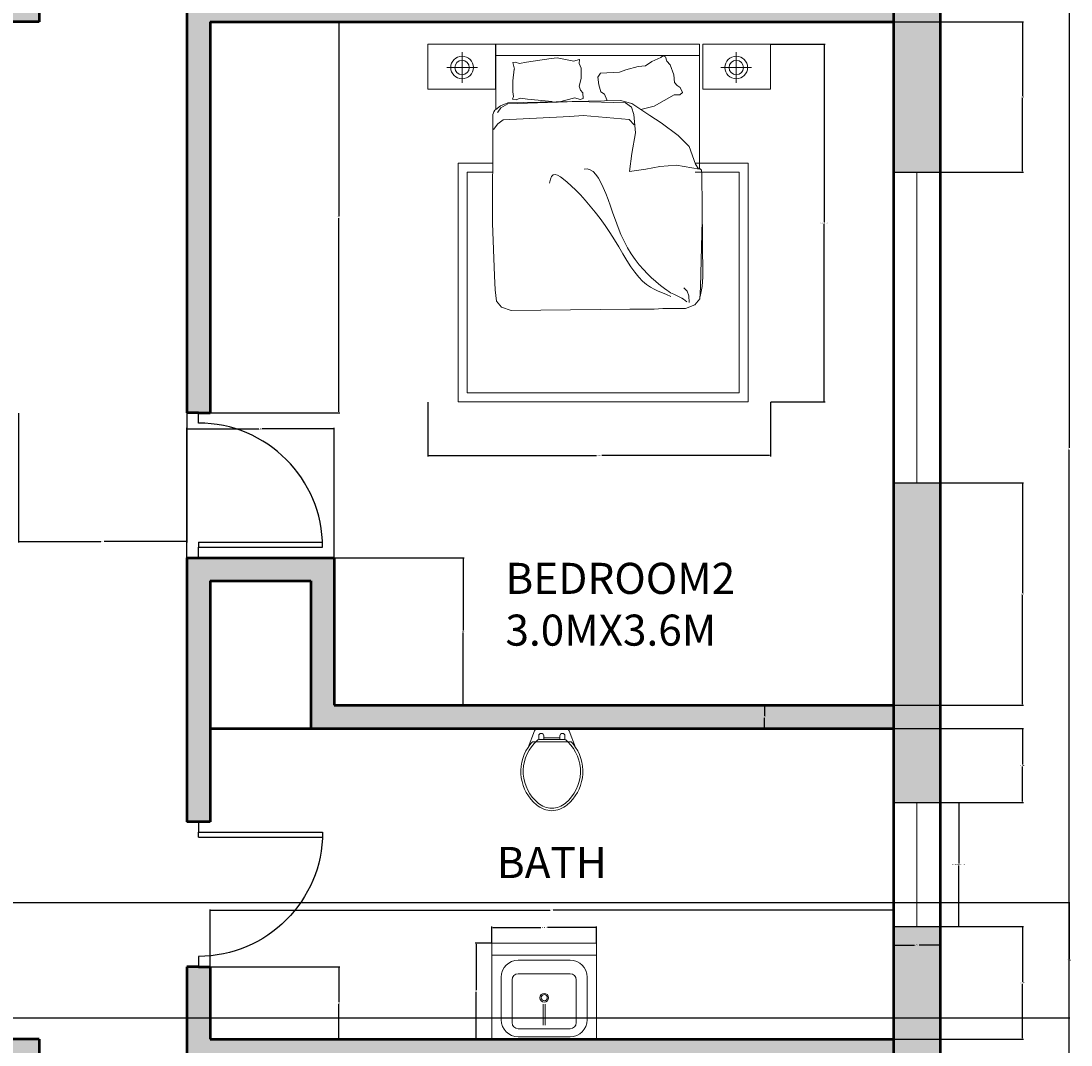
# Model space of a CAD drawing. Units: inches. Extents: x 3 to 380, y -485 to 60.
# Tile 6 of 8: x 177 to 380, y -328 to -130. Entities that reach past the tile are written whole.
import ezdxf

# ---------------------------------------------------------------- set-up
doc = ezdxf.new("R2010")
doc.units = ezdxf.units.IN
doc.header["$MEASUREMENT"] = 0
for name, color, linetype, lineweight in [('A-ANNO-DIMS', 2, 'Continuous', 18), ('A-AREA-IDEN', 7, 'Continuous', 25), ('A-DOOR', 3, 'Continuous', 25), ('A-FLOR-FIXT', 9, 'Continuous', 18), ('A-FURN', 8, 'Continuous', 18), ('A-GLAZ', 4, 'Continuous', 18), ('A-WALL', 7, 'Continuous', 50), ('A-WALL-PATT', 252, 'Continuous', 13)]:
    doc.layers.add(name, color=color, linetype=linetype, lineweight=lineweight)
doc.styles.get("Standard").update_dxf_attribs({"font": 'arial.ttf'})
doc.dimstyles.get("Standard").update_dxf_attribs({"dimtxt": 0.18, "dimasz": 0.18, "dimexe": 0.18, "dimexo": 0.0625, "dimgap": 0.09, "dimtad": 0, "dimtih": 1, "dimtoh": 1, "dimdec": 0, "dimzin": 0, "dimdsep": 46, "dimlunit": 3, "dimtxsty": 'Standard', "dimcen": 0.09, "dimadec": 0, "dimazin": 0, "dimtfac": 1, "dimtdec": 0, "dimtofl": 0, "dimtmove": 0, "dimatfit": 3, "dimfxl": 1, "dimtolj": 1, "dimtzin": 0, "dimarcsym": 0})

# ---------------------------------------------------------------- blocks, each defined once
blk = doc.blocks.new('М14 600х655')
for p, q in [((-655, 600), (-655, 0)), ((-655, 600), (-655, 0)), ((-655, 0), (-655, 600)), ((0, 600), (-655, 600)), ((0, 0), (0, 600)), ((0, 525), (-655, 525)), ((-165.1, 494.1), (-489.9, 494.1)), ((-165.4, 408.4), (-490.2, 408.4)), ((-595.8, 388.1), (-595.8, 121.3)), ((-528.4, 370.1), (-528.4, 103.3)), ((-127.2, 103.3), (-127.2, 370.1)), ((-59.2, 121.3), (-59.2, 388.1)), ((-333.5, 87.1), (-333.5, 219.6)), ((-321.5, 87.1), (-321.5, 219.6)), ((-655, 0), (-655, 0)), ((-655, 0), (-655, 0)), ((-655, 0), (0, 0)), ((-655, 0), (0, 0)), ((-490.2, 65.1), (-165.4, 65.1)), ((-489.9, 15.4), (-165.1, 15.4))]:
    blk.add_line(p, q)
for radius in [27.6, 19.3]:
    blk.add_circle((-327.5, 258.9), radius)
for centre, radius, start, end in [((-489.9, 388.1), 105.9, 90, 180), ((-165.1, 388.1), 105.9, 0, 90), ((-490.2, 370.1), 38.2, 90, 180), ((-165.4, 370.1), 38.2, 0, 90), ((-489.9, 121.3), 105.9, 180, 270), ((-490.2, 103.3), 38.2, 180, 270), ((-165.4, 103.3), 38.2, 270, 0), ((-165.1, 121.3), 105.9, 270, 0)]:
    blk.add_arc(centre, radius, start, end)
blk = doc.blocks.new('BED-DOUBLE-WITH-NIGHTSTANDS')
for p, q in [((13.15, 56.48), (13.15, 69.11)), ((6.62, 67.56), (6.62, 61.62)), ((59.58, 67.56), (59.58, 61.62)), ((16.76, 64.3), (16.42, 65.57)), ((25.02, 66.47), (23.83, 66.33)), ((28.24, 65.8), (25.02, 66.47)), ((29.23, 66.16), (28.24, 65.8)), ((29.33, 66.13), (29.23, 66.16)), ((29.33, 66.13), (29.25, 65.4)), ((29.33, 66.13), (29.25, 65.4)), ((29.25, 65.4), (29.65, 64.45)), ((40.63, 64.79), (42.02, 64.91)), ((42.02, 64.91), (43.24, 65.73)), ((42.02, 64.91), (43.24, 65.73)), ((43.24, 65.73), (44.98, 66.53)), ((46.15, 65.85), (46.84, 65.09)), ((46.84, 65.09), (47.51, 63.2)), ((3.65, 64.59), (9.59, 64.59)), ((29.65, 64.45), (29.63, 62.44)), ((33.33, 63.47), (37.02, 63.69)), ((37.02, 63.69), (38.27, 64.16)), ((38.27, 64.16), (40.63, 64.79)), ((47.51, 63.2), (47.67, 61.68)), ((62.55, 64.59), (56.61, 64.59)), ((29.63, 62.44), (29.27, 60.96)), ((29.27, 60.96), (29.52, 60.24)), ((47.67, 61.68), (48.15, 61.09)), ((48.15, 61.09), (48.75, 60.71)), ((29.52, 60.24), (29.96, 59.68)), ((29.96, 59.68), (30.03, 58.63)), ((47.6, 59.3), (43.73, 57.13)), ((48.66, 59.34), (47.6, 59.3)), ((49.17, 59.74), (48.66, 59.34)), ((48.75, 60.71), (49.17, 59.74)), ((28.4, 58.75), (25.21, 57.93)), ((29.41, 58.43), (28.4, 58.75)), ((30.03, 58.63), (29.41, 58.43)), ((12.59, 55.61), (12.54, 55)), ((12.54, 55), (12.56, 53.58)), ((12.56, 53.58), (12.48, 34.55)), ((52.39, 45), (52.46, 45.03)), ((52.97, 37.68), (52.91, 43.85)), ((53.11, 24.16), (52.97, 37.68)), ((12.48, 34.55), (12.89, 24.35)), ((53.02, 35.03), (52.75, 24.82)), ((12.89, 24.35), (13.03, 21.68)), ((52.75, 24.82), (52.69, 22.14)), ((53, 22.29), (53.11, 24.16)), ((13.03, 21.68), (13.27, 19.48)), ((50.1, 21.39), (49.46, 22.06)), ((50.39, 20.5), (50.1, 21.39)), ((50.45, 19.2), (50.39, 20.5)), ((52.69, 22.14), (52.52, 19.94)), ((52.63, 20.34), (53, 22.29)), ((13.27, 19.48), (14.23, 18.32)), ((14.23, 18.32), (16.09, 17.69)), ((51.59, 18.75), (49.75, 18.06)), ((52.52, 19.94), (51.59, 18.75)), ((39.03, 17.94), (16.09, 17.69)), ((39.03, 17.94), (43.71, 17.94)), ((43.71, 17.94), (45.37, 18.06)), ((45.37, 18.06), (49.75, 18.06))]:
    blk.add_line(p, q)
for points in [[(0, 60.38), (13.1, 60.38), (13.1, 69.11), (0, 69.11)], [(66.2, 60.38), (53.1, 60.38), (53.1, 69.11), (66.2, 69.11)]]:
    blk.add_lwpolyline(points, close=True)
for points in [[(13.15, 69.11), (52.45, 69.11), (52.45, 45.06)], [(52.45, 66.93), (13.15, 66.93)], [(23.83, 66.33), (19.08, 65.62), (17.7, 65.39), (16.88, 65.65), (16.42, 65.57)], [(46.15, 65.85), (45.9, 66.66), (45.38, 66.82), (44.98, 66.53)], [(24.02, 58.01), (19.24, 58.51), (17.85, 58.68), (17.04, 58.38), (16.37, 58.47), (16.56, 59), (16.45, 59.9), (16.42, 62), (16.71, 64.3)], [(33.33, 63.47), (32.82, 62.74), (33.06, 61.23), (33.43, 59.89), (34.16, 59.47), (34.58, 58.37), (34.59, 58.17)], [(52.45, 44.97), (48.05, 45.75), (44.8, 45.5), (42.14, 44.97), (38.99, 44.52), (39.41, 47.96), (40.12, 51.96), (39.81, 55.5), (39.35, 56.93), (38.2, 57.74), (28.88, 58), (15.49, 57.6), (14.12, 56.79), (13.54, 55.99), (13.47, 55.91)], [(13.48, 56.71), (14.02, 57.18), (15.49, 57.8), (37.2, 58.22), (39.38, 57.66), (42.87, 55.35), (45.06, 53.9), (48.36, 51.48), (50.46, 49.34), (51.7, 45.9), (52.31, 45)], [(43.73, 57.13), (41.15, 56.49)], [(12.61, 55.65), (12.74, 56.06), (12.92, 56.37), (13.15, 56.48), (13.4, 56.7), (13.44, 56.72)], [(39.86, 53.54), (38.87, 54.55), (30.01, 55.3), (27.42, 55.15), (14.59, 54.51), (13.51, 53.69), (12.69, 52.6)], [(51.61, 46.15), (61.88, 46.15), (61.88, 0), (5.85, 0), (5.85, 46.15), (12.53, 46.15)], [(50.06, 19.34), (49.7, 19.62), (49.37, 19.84), (49.06, 20.03), (48.78, 20.19), (48.52, 20.33), (48.27, 20.44), (48.02, 20.55), (47.76, 20.67), (47.5, 20.79), (47.21, 20.93), (46.9, 21.1), (46.56, 21.31), (46.16, 21.57), (45.71, 21.89), (45.2, 22.29), (44.61, 22.76), (43.95, 23.32), (43.23, 23.98), (42.45, 24.72), (41.66, 25.56), (40.85, 26.48), (40.05, 27.49), (39.29, 28.58), (38.57, 29.76), (37.91, 31.03), (37.31, 32.35), (36.75, 33.71), (36.24, 35.08), (35.75, 36.45), (35.28, 37.79), (34.82, 39.08), (34.36, 40.29), (33.9, 41.4), (33.43, 42.39), (32.94, 43.25), (32.44, 43.96), (31.91, 44.5), (31.37, 44.86), (30.8, 45.01), (30.2, 44.94)], [(52.91, 43.91), (52.84, 44.76), (52.6, 45.01), (52.45, 45.06)], [(51.61, 44.4), (60.14, 44.4), (60.14, 1.75), (7.59, 1.75), (7.59, 44.4), (12.53, 44.4)], [(46.96, 20.37), (46.12, 20.73), (45.31, 21.07), (44.52, 21.41), (43.75, 21.77), (42.99, 22.2), (42.24, 22.71), (41.49, 23.33), (40.74, 24.1), (39.99, 25.04), (39.23, 26.12), (38.46, 27.32), (37.67, 28.61), (36.87, 29.96), (36.03, 31.34), (35.16, 32.73), (34.26, 34.09), (33.32, 35.4), (32.36, 36.66), (31.39, 37.84), (30.42, 38.95), (29.48, 39.98), (28.57, 40.91), (27.72, 41.73), (26.93, 42.45), (26.23, 43.05), (25.61, 43.51), (25.06, 43.81), (24.6, 43.93), (24.22, 43.85), (23.91, 43.56), (23.68, 43.04), (23.52, 42.25)]]:
    blk.add_lwpolyline(points)
for centre, radius in [((6.62, 64.59), 2.18), ((6.62, 64.59), 1.4), ((59.58, 64.59), 2.18), ((59.58, 64.59), 1.4)]:
    blk.add_circle(centre, radius)
blk = doc.blocks.new('WC-PLAN')
for p, q in [((2.25, 13.31), (2.91, 13.31)), ((2.91, 13.31), (5.99, 13.31)), ((9.08, 13.31), (5.99, 13.31)), ((9.08, 13.31), (9.73, 13.31))]:
    blk.add_line(p, q)
for points in [[(5.99, 15.68), (3, 15.68, 0.31031), (2.63, 15.43), (1.4, 12.23, 0.209071)], [(3.45, 13.78), (3.45, 14.44, -1), (4.45, 14.44), (4.45, 14.1)], [(5.99, 15.68), (8.98, 15.68, -0.31031), (9.35, 15.43), (10.58, 12.23, -0.209071)], [(8.53, 13.78), (8.53, 14.44, 1), (7.53, 14.44), (7.53, 14.1)], [(1.4, 12.23, 0.383919), (3.04, 1.13, 0.163732), (5.99, 0, 0.359733)], [(2.59, 12.99, 0.431639), (3.34, 1.49, 0.162618), (5.99, 0.47, 0.470877)], [(2.25, 13.31, 0.040937), (1.4, 12.23, 0.163732)], [(2.91, 13.31, 0.014165), (2.59, 12.99, 0.162618)], [(3.45, 13.78, 0.022712), (2.91, 13.31, 0.162618)], [(5.99, 13.78), (3.45, 13.78, 0.022712)], [(5.99, 13.78), (8.53, 13.78, -0.476108)], [(9.08, 13.31, -0.448546), (8.64, 1.49, -0.162618), (5.99, 0.47, -0.470877)], [(10.58, 12.23, -0.383919), (8.94, 1.13, -0.163732), (5.99, 0, -0.359733)], [(8.53, 13.78, -0.022712), (9.08, 13.31, -0.162618)], [(9.73, 13.31, -0.040937), (10.58, 12.23, -0.163732)]]:
    blk.add_lwpolyline(points, format="xyb")
for points in [[(7.53, 14.1), (4.45, 14.1)], [(4.45, 14.1), (4.45, 13.78)], [(7.53, 14.1), (7.53, 13.78)]]:
    blk.add_lwpolyline(points)
blk = doc.blocks.new('WIN-60X9')
for p, q in [((60, 9), (0, 9)), ((0, 9), (0, 0)), ((60, 0), (60, 9)), ((0, 4.5), (60, 4.5)), ((0, 0), (60, 0))]:
    blk.add_line(p, q)
blk = doc.blocks.new('WIN-24X9')
for p, q in [((0, 24), (0, 0)), ((9, 24), (0, 24)), ((4.5, 24), (4.5, 0)), ((9, 0), (9, 24)), ((0, 0), (9, 0))]:
    blk.add_line(p, q)
blk = doc.blocks.new('DOOR-SWING-24')
for p, q in [((25, 0), (25, 24)), ((26, 0), (26, 24)), ((2, 0), (0, 0)), ((25, 0), (26, 0)), ((28, 0), (26, 0))]:
    blk.add_line(p, q)
blk.add_arc((26, 0), 24, 90, 180)
blk = doc.blocks.new('*D21')
at = {"layer": 'A-ANNO-DIMS', "color": 0, "lineweight": -2, "transparency": 16777216}
for p, q in [((354.9, -281.1), (358.62, -281.1)), ((358.44, -281.28), (358.44, -292.92)), ((358.44, -304.92), (358.44, -293.28)), ((354.9, -305.1), (358.62, -305.1))]:
    blk.add_line(p, q, dxfattribs=at)
at = {"layer": 'A-ANNO-DIMS', "color": 0, "transparency": 16777216}
for points in [[(358.41, -281.28), (358.47, -281.28), (358.44, -281.1)], [(358.41, -304.92), (358.47, -304.92), (358.44, -305.1)]]:
    blk.add_solid(points, dxfattribs=at)
at = {"layer": 'Defpoints', "color": 0, "transparency": 16777216}
for p in [(354.84, -281.1), (358.44, -281.1), (354.84, -305.1)]:
    blk.add_point(p, dxfattribs=at)
at = {"layer": 'A-ANNO-DIMS', "color": 0, "transparency": 16777216, "insert": (358.44, -293.1), "char_height": 0.18, "attachment_point": 5}
blk.add_mtext('\\A1;BATH WINDOW 24 TYP.', dxfattribs=at)
blk = doc.blocks.new('*D22')
at = {"layer": 'A-ANNO-DIMS', "color": 0, "lineweight": -2, "transparency": 16777216}
for p, q in [((345.84, -305.16), (345.84, -308.88)), ((354.84, -305.16), (354.84, -308.88)), ((346.02, -308.7), (349.88, -308.7)), ((354.66, -308.7), (350.8, -308.7))]:
    blk.add_line(p, q, dxfattribs=at)
at = {"layer": 'A-ANNO-DIMS', "color": 0, "transparency": 16777216}
for points in [[(346.02, -308.67), (346.02, -308.73), (345.84, -308.7)], [(354.66, -308.67), (354.66, -308.73), (354.84, -308.7)]]:
    blk.add_solid(points, dxfattribs=at)
at = {"layer": 'Defpoints', "color": 0, "transparency": 16777216}
for p in [(345.84, -305.1), (354.84, -305.1), (354.84, -308.7)]:
    blk.add_point(p, dxfattribs=at)
at = {"layer": 'A-ANNO-DIMS', "color": 0, "transparency": 16777216, "insert": (350.34, -308.7), "char_height": 0.18, "attachment_point": 5}
blk.add_mtext('\\A1;9 TYP.', dxfattribs=at)
blk = doc.blocks.new('*D27')
at = {"layer": 'A-ANNO-DIMS', "color": 0, "lineweight": -2, "transparency": 16777216}
for p, q in [((322.16, -134.65), (332.64, -134.65)), ((332.46, -134.83), (332.46, -169.02)), ((332.46, -203.58), (332.46, -169.38)), ((322.16, -203.76), (332.64, -203.76))]:
    blk.add_line(p, q, dxfattribs=at)
at = {"layer": 'A-ANNO-DIMS', "color": 0, "transparency": 16777216}
for points in [[(332.43, -134.83), (332.49, -134.83), (332.46, -134.65)], [(332.43, -203.58), (332.49, -203.58), (332.46, -203.76)]]:
    blk.add_solid(points, dxfattribs=at)
at = {"layer": 'Defpoints', "color": 0, "transparency": 16777216}
for p in [(322.1, -134.65), (332.46, -134.65), (322.1, -203.76)]:
    blk.add_point(p, dxfattribs=at)
at = {"layer": 'A-ANNO-DIMS', "color": 0, "transparency": 16777216, "insert": (332.46, -169.2), "char_height": 0.18, "attachment_point": 5}
blk.add_mtext('\\A1;BED GROUP 69 TYP.', dxfattribs=at)
blk = doc.blocks.new('*D28')
at = {"layer": 'A-ANNO-DIMS', "color": 0, "lineweight": -2, "transparency": 16777216}
for p, q in [((255.9, -203.82), (255.9, -214.3)), ((322.1, -203.82), (322.1, -214.3)), ((256.08, -214.12), (288.47, -214.12)), ((321.92, -214.12), (289.52, -214.12))]:
    blk.add_line(p, q, dxfattribs=at)
at = {"layer": 'A-ANNO-DIMS', "color": 0, "transparency": 16777216}
for points in [[(256.08, -214.09), (256.08, -214.15), (255.9, -214.12)], [(321.92, -214.09), (321.92, -214.15), (322.1, -214.12)]]:
    blk.add_solid(points, dxfattribs=at)
at = {"layer": 'Defpoints', "color": 0, "transparency": 16777216}
for p in [(255.9, -203.76), (322.1, -203.76), (322.1, -214.12)]:
    blk.add_point(p, dxfattribs=at)
at = {"layer": 'A-ANNO-DIMS', "color": 0, "transparency": 16777216, "insert": (289, -214.12), "char_height": 0.18, "attachment_point": 5}
blk.add_mtext('\\A1;66 TYP.', dxfattribs=at)
blk = doc.blocks.new('*D35')
at = {"layer": 'A-ANNO-DIMS', "color": 0, "lineweight": -2, "transparency": 16777216}
for p, q in [((268.27, -308.23), (268.27, -305.08)), ((268.45, -305.26), (277.76, -305.26)), ((288.33, -305.26), (279.01, -305.26)), ((288.51, -308.23), (288.51, -305.08))]:
    blk.add_line(p, q, dxfattribs=at)
at = {"layer": 'A-ANNO-DIMS', "color": 0, "transparency": 16777216}
for points in [[(268.45, -305.23), (268.45, -305.29), (268.27, -305.26)], [(288.33, -305.23), (288.33, -305.29), (288.51, -305.26)]]:
    blk.add_solid(points, dxfattribs=at)
at = {"layer": 'Defpoints', "color": 0, "transparency": 16777216}
for p in [(288.51, -305.26), (268.27, -308.29), (288.51, -308.29)]:
    blk.add_point(p, dxfattribs=at)
at = {"layer": 'A-ANNO-DIMS', "color": 0, "transparency": 16777216, "insert": (278.39, -305.26), "char_height": 0.18, "attachment_point": 5}
blk.add_mtext('\\A1;BASIN 20', dxfattribs=at)
blk = doc.blocks.new('*D36')
at = {"layer": 'A-ANNO-DIMS', "color": 0, "lineweight": -2, "transparency": 16777216}
for p, q in [((268.2, -308.29), (265.05, -308.29)), ((265.23, -308.47), (265.23, -317.38)), ((265.23, -326.66), (265.23, -317.75)), ((268.2, -326.84), (265.05, -326.84))]:
    blk.add_line(p, q, dxfattribs=at)
at = {"layer": 'A-ANNO-DIMS', "color": 0, "transparency": 16777216}
for points in [[(265.2, -308.47), (265.26, -308.47), (265.23, -308.29)], [(265.2, -326.66), (265.26, -326.66), (265.23, -326.84)]]:
    blk.add_solid(points, dxfattribs=at)
at = {"layer": 'Defpoints', "color": 0, "transparency": 16777216}
for p in [(265.23, -308.29), (268.27, -308.29), (268.27, -326.84)]:
    blk.add_point(p, dxfattribs=at)
at = {"layer": 'A-ANNO-DIMS', "color": 0, "transparency": 16777216, "insert": (265.23, -317.56), "char_height": 0.18, "attachment_point": 5}
blk.add_mtext('\\A1;19', dxfattribs=at)
blk = doc.blocks.new('*D51')
at = {"layer": 'A-ANNO-DIMS', "color": 0, "lineweight": -2, "transparency": 16777216}
for p, q in [((151.9, 34.66), (379.92, 34.66)), ((379.74, 34.48), (379.74, -212.65)), ((379.74, -460.16), (379.74, -213.02)), ((354.9, -460.34), (379.92, -460.34))]:
    blk.add_line(p, q, dxfattribs=at)
at = {"layer": 'A-ANNO-DIMS', "color": 0, "transparency": 16777216}
for points in [[(379.71, 34.48), (379.77, 34.48), (379.74, 34.66)], [(379.71, -460.16), (379.77, -460.16), (379.74, -460.34)]]:
    blk.add_solid(points, dxfattribs=at)
at = {"layer": 'Defpoints', "color": 0, "transparency": 16777216}
for p in [(151.84, 34.66), (354.84, -460.34), (379.74, -460.34)]:
    blk.add_point(p, dxfattribs=at)
at = {"layer": 'A-ANNO-DIMS', "color": 0, "transparency": 16777216, "insert": (379.74, -212.84), "char_height": 0.18, "attachment_point": 5}
blk.add_mtext('\\A1;495', dxfattribs=at)
blk = doc.blocks.new('*D64')
at = {"layer": 'A-ANNO-DIMS', "color": 0, "lineweight": -2, "transparency": 16777216}
for p, q in [((345.9, -130.34), (370.92, -130.34)), ((370.74, -130.52), (370.74, -144.67)), ((370.74, -159.19), (370.74, -145.04)), ((345.9, -159.37), (370.92, -159.37))]:
    blk.add_line(p, q, dxfattribs=at)
at = {"layer": 'A-ANNO-DIMS', "color": 0, "transparency": 16777216}
for points in [[(370.71, -130.52), (370.77, -130.52), (370.74, -130.34)], [(370.71, -159.19), (370.77, -159.19), (370.74, -159.37)]]:
    blk.add_solid(points, dxfattribs=at)
at = {"layer": 'Defpoints', "color": 0, "transparency": 16777216}
for p in [(345.84, -130.34), (345.84, -159.37), (370.74, -159.37)]:
    blk.add_point(p, dxfattribs=at)
at = {"layer": 'A-ANNO-DIMS', "color": 0, "transparency": 16777216, "insert": (370.74, -144.85), "char_height": 0.18, "attachment_point": 5}
blk.add_mtext('\\A1;29.04', dxfattribs=at)
blk = doc.blocks.new('*D65')
at = {"layer": 'A-ANNO-DIMS', "color": 0, "lineweight": -2, "transparency": 16777216}
for p, q in [((345.9, -219.37), (370.92, -219.37)), ((370.74, -219.55), (370.74, -240.67)), ((370.74, -262.16), (370.74, -241.04)), ((345.9, -262.34), (370.92, -262.34))]:
    blk.add_line(p, q, dxfattribs=at)
at = {"layer": 'A-ANNO-DIMS', "color": 0, "transparency": 16777216}
for points in [[(370.71, -219.55), (370.77, -219.55), (370.74, -219.37)], [(370.71, -262.16), (370.77, -262.16), (370.74, -262.34)]]:
    blk.add_solid(points, dxfattribs=at)
at = {"layer": 'Defpoints', "color": 0, "transparency": 16777216}
for p in [(345.84, -219.37), (345.84, -262.34), (370.74, -262.34)]:
    blk.add_point(p, dxfattribs=at)
at = {"layer": 'A-ANNO-DIMS', "color": 0, "transparency": 16777216, "insert": (370.74, -240.85), "char_height": 0.18, "attachment_point": 5}
blk.add_mtext('\\A1;42.96', dxfattribs=at)
blk = doc.blocks.new('*D66')
at = {"layer": 'A-ANNO-DIMS', "color": 0, "lineweight": -2, "transparency": 16777216}
for p, q in [((345.9, -266.84), (370.92, -266.84)), ((370.74, -267.02), (370.74, -273.79)), ((370.74, -280.92), (370.74, -274.15)), ((345.9, -281.1), (370.92, -281.1))]:
    blk.add_line(p, q, dxfattribs=at)
at = {"layer": 'A-ANNO-DIMS', "color": 0, "transparency": 16777216}
for points in [[(370.71, -267.02), (370.77, -267.02), (370.74, -266.84)], [(370.71, -280.92), (370.77, -280.92), (370.74, -281.1)]]:
    blk.add_solid(points, dxfattribs=at)
at = {"layer": 'Defpoints', "color": 0, "transparency": 16777216}
for p in [(345.84, -266.84), (345.84, -281.1), (370.74, -281.1)]:
    blk.add_point(p, dxfattribs=at)
at = {"layer": 'A-ANNO-DIMS', "color": 0, "transparency": 16777216, "insert": (370.74, -273.97), "char_height": 0.18, "attachment_point": 5}
blk.add_mtext('\\A1;14.265', dxfattribs=at)
blk = doc.blocks.new('*D67')
at = {"layer": 'A-ANNO-DIMS', "color": 0, "lineweight": -2, "transparency": 16777216}
for p, q in [((345.9, -305.1), (370.92, -305.1)), ((370.74, -305.28), (370.74, -315.79)), ((370.74, -326.66), (370.74, -316.15)), ((345.9, -326.84), (370.92, -326.84))]:
    blk.add_line(p, q, dxfattribs=at)
at = {"layer": 'A-ANNO-DIMS', "color": 0, "transparency": 16777216}
for points in [[(370.71, -305.28), (370.77, -305.28), (370.74, -305.1)], [(370.71, -326.66), (370.77, -326.66), (370.74, -326.84)]]:
    blk.add_solid(points, dxfattribs=at)
at = {"layer": 'Defpoints', "color": 0, "transparency": 16777216}
for p in [(345.84, -305.1), (345.84, -326.84), (370.74, -326.84)]:
    blk.add_point(p, dxfattribs=at)
at = {"layer": 'A-ANNO-DIMS', "color": 0, "transparency": 16777216, "insert": (370.74, -315.97), "char_height": 0.18, "attachment_point": 5}
blk.add_mtext('\\A1;21.735', dxfattribs=at)
blk = doc.blocks.new('*D77')
at = {"layer": 'A-ANNO-DIMS', "color": 0, "lineweight": -2, "transparency": 16777216}
for p, q in [((213.9, -130.34), (238.92, -130.34)), ((238.74, -130.52), (238.74, -167.9)), ((238.74, -205.66), (238.74, -168.27)), ((213.9, -205.84), (238.92, -205.84))]:
    blk.add_line(p, q, dxfattribs=at)
at = {"layer": 'A-ANNO-DIMS', "color": 0, "transparency": 16777216}
for points in [[(238.71, -130.52), (238.77, -130.52), (238.74, -130.34)], [(238.71, -205.66), (238.77, -205.66), (238.74, -205.84)]]:
    blk.add_solid(points, dxfattribs=at)
at = {"layer": 'Defpoints', "color": 0, "transparency": 16777216}
for p in [(213.84, -130.34), (213.84, -205.84), (238.74, -205.84)]:
    blk.add_point(p, dxfattribs=at)
at = {"layer": 'A-ANNO-DIMS', "color": 0, "transparency": 16777216, "insert": (238.74, -168.09), "char_height": 0.18, "attachment_point": 5}
blk.add_mtext('\\A1;75.5', dxfattribs=at)
blk = doc.blocks.new('*D78')
at = {"layer": 'A-ANNO-DIMS', "color": 0, "lineweight": -2, "transparency": 16777216}
for p, q in [((213.84, -326.77), (213.84, -301.76)), ((214.02, -301.94), (279.56, -301.94)), ((345.66, -301.94), (280.12, -301.94)), ((345.84, -326.77), (345.84, -301.76))]:
    blk.add_line(p, q, dxfattribs=at)
at = {"layer": 'A-ANNO-DIMS', "color": 0, "transparency": 16777216}
for points in [[(214.02, -301.91), (214.02, -301.97), (213.84, -301.94)], [(345.66, -301.91), (345.66, -301.97), (345.84, -301.94)]]:
    blk.add_solid(points, dxfattribs=at)
at = {"layer": 'Defpoints', "color": 0, "transparency": 16777216}
for p in [(345.84, -301.94), (213.84, -326.84), (345.84, -326.84)]:
    blk.add_point(p, dxfattribs=at)
at = {"layer": 'A-ANNO-DIMS', "color": 0, "transparency": 16777216, "insert": (279.84, -301.94), "char_height": 0.18, "attachment_point": 5}
blk.add_mtext('\\A1;132', dxfattribs=at)
blk = doc.blocks.new('*D79')
at = {"layer": 'A-ANNO-DIMS', "color": 0, "lineweight": -2, "transparency": 16777216}
for p, q in [((213.9, -312.84), (238.92, -312.84)), ((238.74, -313.02), (238.74, -319.66)), ((238.74, -326.66), (238.74, -320.02)), ((213.9, -326.84), (238.92, -326.84))]:
    blk.add_line(p, q, dxfattribs=at)
at = {"layer": 'A-ANNO-DIMS', "color": 0, "transparency": 16777216}
for points in [[(238.71, -313.02), (238.77, -313.02), (238.74, -312.84)], [(238.71, -326.66), (238.77, -326.66), (238.74, -326.84)]]:
    blk.add_solid(points, dxfattribs=at)
at = {"layer": 'Defpoints', "color": 0, "transparency": 16777216}
for p in [(213.84, -312.84), (213.84, -326.84), (238.74, -326.84)]:
    blk.add_point(p, dxfattribs=at)
at = {"layer": 'A-ANNO-DIMS', "color": 0, "transparency": 16777216, "insert": (238.74, -319.84), "char_height": 0.18, "attachment_point": 5}
blk.add_mtext('\\A1;14', dxfattribs=at)
blk = doc.blocks.new('*D83')
at = {"layer": 'A-ANNO-DIMS', "color": 0, "lineweight": -2, "transparency": 16777216}
for p, q in [((345.78, -262.34), (320.76, -262.34)), ((320.94, -262.52), (320.94, -264.4)), ((320.94, -266.66), (320.94, -264.77)), ((345.78, -266.84), (320.76, -266.84))]:
    blk.add_line(p, q, dxfattribs=at)
at = {"layer": 'A-ANNO-DIMS', "color": 0, "transparency": 16777216}
for points in [[(320.91, -262.52), (320.97, -262.52), (320.94, -262.34)], [(320.91, -266.66), (320.97, -266.66), (320.94, -266.84)]]:
    blk.add_solid(points, dxfattribs=at)
at = {"layer": 'Defpoints', "color": 0, "transparency": 16777216}
for p in [(320.94, -262.34), (345.84, -262.34), (345.84, -266.84)]:
    blk.add_point(p, dxfattribs=at)
at = {"layer": 'A-ANNO-DIMS', "color": 0, "transparency": 16777216, "insert": (320.94, -264.59), "char_height": 0.18, "attachment_point": 5}
blk.add_mtext('\\A1;4.5', dxfattribs=at)
blk = doc.blocks.new('*D84')
at = {"layer": 'A-ANNO-DIMS', "color": 0, "lineweight": -2, "transparency": 16777216}
for p, q in [((209.34, -233.77), (209.34, -208.76)), ((237.84, -233.77), (237.84, -208.76)), ((209.52, -208.94), (223.26, -208.94)), ((237.66, -208.94), (223.92, -208.94))]:
    blk.add_line(p, q, dxfattribs=at)
at = {"layer": 'A-ANNO-DIMS', "color": 0, "transparency": 16777216}
for points in [[(209.52, -208.91), (209.52, -208.97), (209.34, -208.94)], [(237.66, -208.91), (237.66, -208.97), (237.84, -208.94)]]:
    blk.add_solid(points, dxfattribs=at)
at = {"layer": 'Defpoints', "color": 0, "transparency": 16777216}
for p in [(237.84, -208.94), (209.34, -233.84), (237.84, -233.84)]:
    blk.add_point(p, dxfattribs=at)
at = {"layer": 'A-ANNO-DIMS', "color": 0, "transparency": 16777216, "insert": (223.59, -208.94), "char_height": 0.18, "attachment_point": 5}
blk.add_mtext('\\A1;28.5', dxfattribs=at)
blk = doc.blocks.new('*D85')
at = {"layer": 'A-ANNO-DIMS', "color": 0, "lineweight": -2, "transparency": 16777216}
for p, q in [((237.9, -233.84), (262.92, -233.84)), ((262.74, -234.02), (262.74, -247.9)), ((262.74, -262.16), (262.74, -248.27)), ((237.9, -262.34), (262.92, -262.34))]:
    blk.add_line(p, q, dxfattribs=at)
at = {"layer": 'A-ANNO-DIMS', "color": 0, "transparency": 16777216}
for points in [[(262.71, -234.02), (262.77, -234.02), (262.74, -233.84)], [(262.71, -262.16), (262.77, -262.16), (262.74, -262.34)]]:
    blk.add_solid(points, dxfattribs=at)
at = {"layer": 'Defpoints', "color": 0, "transparency": 16777216}
for p in [(237.84, -233.84), (237.84, -262.34), (262.74, -262.34)]:
    blk.add_point(p, dxfattribs=at)
at = {"layer": 'A-ANNO-DIMS', "color": 0, "transparency": 16777216, "insert": (262.74, -248.09), "char_height": 0.18, "attachment_point": 5}
blk.add_mtext('\\A1;28.5', dxfattribs=at)
blk = doc.blocks.new('*D86')
at = {"layer": 'A-ANNO-DIMS', "color": 0, "lineweight": -2, "transparency": 16777216}
for p, q in [((176.84, -205.9), (176.84, -230.92)), ((209.34, -205.9), (209.34, -230.92)), ((177.02, -230.74), (192.77, -230.74)), ((209.16, -230.74), (193.41, -230.74))]:
    blk.add_line(p, q, dxfattribs=at)
at = {"layer": 'A-ANNO-DIMS', "color": 0, "transparency": 16777216}
for points in [[(177.02, -230.71), (177.02, -230.77), (176.84, -230.74)], [(209.16, -230.71), (209.16, -230.77), (209.34, -230.74)]]:
    blk.add_solid(points, dxfattribs=at)
at = {"layer": 'Defpoints', "color": 0, "transparency": 16777216}
for p in [(176.84, -205.84), (209.34, -205.84), (176.84, -230.74)]:
    blk.add_point(p, dxfattribs=at)
at = {"layer": 'A-ANNO-DIMS', "color": 0, "transparency": 16777216, "insert": (193.09, -230.74), "char_height": 0.18, "attachment_point": 5}
blk.add_mtext('\\A1;32.5', dxfattribs=at)
blk = doc.blocks.new('*D99')
at = {"layer": 'A-ANNO-DIMS', "color": 0, "lineweight": -2, "transparency": 16777216}
for p, q in [((76.32, -300.46), (379.92, -300.46)), ((379.74, -300.64), (379.74, -311.4)), ((379.74, -322.52), (379.74, -311.76)), ((76.32, -322.7), (379.92, -322.7))]:
    blk.add_line(p, q, dxfattribs=at)
at = {"layer": 'A-ANNO-DIMS', "color": 0, "transparency": 16777216}
for points in [[(379.71, -300.64), (379.77, -300.64), (379.74, -300.46)], [(379.71, -322.52), (379.77, -322.52), (379.74, -322.7)]]:
    blk.add_solid(points, dxfattribs=at)
at = {"layer": 'Defpoints', "color": 0, "transparency": 16777216}
for p in [(76.25, -300.46), (76.25, -322.7), (379.74, -322.7)]:
    blk.add_point(p, dxfattribs=at)
at = {"layer": 'A-ANNO-DIMS', "color": 0, "transparency": 16777216, "insert": (379.74, -311.58), "char_height": 0.18, "attachment_point": 5}
blk.add_mtext('\\A1;22.236', dxfattribs=at)

msp = doc.modelspace()

# ---------------------------------------------------------------- hatches: boundary and pattern name
at = {"layer": 'A-WALL-PATT'}
h = msp.add_hatch(color=256, dxfattribs=at)
h.dxf.hatch_style = 1
h.paths.add_polyline_path([(36.8404, 6.1643), (51.3404, 6.1643), (51.3404, 15.1643), (27.8404, 15.1643), (27.8404, -143.6318), (36.8404, -143.6318)])
h.paths.add_polyline_path([(125.8404, 10.6643), (125.8404, 15.1643), (111.3404, 15.1643), (111.3404, 6.1643), (125.8404, 6.1643)])
h.paths.add_polyline_path([(170.6358, 15.1643), (153.8404, 15.1643), (153.8404, 6.1643), (156.8404, 6.1643), (156.8404, -82.3357), (173.3404, -82.3357), (173.3404, -130.3357), (177.8404, -130.3357), (180.8404, -130.3357), (180.8404, -125.8357), (177.8404, -125.8357), (177.8404, -82.3357), (201.8404, -82.3357), (201.8404, -38.0857), (197.3404, -38.0857), (197.3404, -77.8357), (161.3404, -77.8357), (161.3404, 6.1643), (170.6358, 6.1643)])
h.paths.add_polyline_path([(241.3739, 15.1643), (194.6358, 15.1643), (194.6358, 6.1643), (241.3739, 6.1643)])
h.paths.add_polyline_path([(201.8404, 6.1643), (197.3404, 6.1643), (197.3404, -12.1977), (201.8404, -12.1977)], flags=17)
h.paths.add_polyline_path([(354.8404, 15.1643), (301.3739, 15.1643), (301.3739, 6.1643), (345.8404, 6.1643), (345.8404, -34.0336), (354.8404, -34.0336)])
h.paths.add_polyline_path([(354.8404, -94.0336), (345.8404, -94.0336), (345.8404, -159.3738), (354.8404, -159.3738)])
h.paths.add_polyline_path([(345.8404, -125.8357), (209.3404, -125.8357), (209.3404, -205.8357), (211.5904, -205.8357), (213.8404, -205.8357), (213.8404, -130.3357), (345.8404, -130.3357)])
h.paths.add_polyline_path([(36.8404, -203.6318), (27.8404, -203.6318), (27.8404, -270.1269), (36.8404, -270.1269)])
h.paths.add_polyline_path([(36.8404, -330.1269), (27.8404, -330.1269), (27.8404, -362.428), (57.3404, -362.428), (57.3404, -353.428), (36.8404, -353.428)])
h.paths.add_polyline_path([(177.8404, -331.3357), (180.8404, -331.3357), (180.8404, -326.8357), (173.3404, -326.8357), (173.3404, -353.428), (165.8404, -353.428), (165.8404, -362.428), (168.8404, -362.428), (168.8404, -451.3357), (168.8404, -460.3357), (231.8404, -460.3357), (231.8404, -451.3357), (177.8404, -451.3357)])
h.paths.add_polyline_path([(354.8404, -305.1003), (345.8404, -305.1003), (345.8404, -363.2829), (354.8404, -363.2829)])
h.paths.add_polyline_path([(345.8404, -326.8357), (213.8404, -326.8357), (213.8404, -312.8357), (211.5904, -312.8357), (209.3404, -312.8357), (209.3404, -331.3357), (345.8404, -331.3357)])
h.paths.add_polyline_path([(345.8404, -262.3357), (237.8404, -262.3357), (237.8404, -233.8357), (209.3404, -233.8357), (209.3404, -284.8357), (213.8404, -284.8357), (213.8404, -238.3357), (233.3404, -238.3357), (233.3404, -266.8357), (345.8404, -266.8357)])
h.paths.add_polyline_path([(354.8404, -219.3738), (345.8404, -219.3738), (345.8404, -281.1003), (354.8404, -281.1003)])

# ---------------------------------------------------------------- linework, layer by layer
at = {"layer": 'A-WALL'}
for p, q in [((354.8404, 15.1643), (354.8404, -460.3357)), ((345.8404, 6.1643), (345.8404, -451.3357)), ((180.8404, -125.8357), (180.8404, -130.3357)), ((209.3404, -125.8357), (209.3404, -205.8357)), ((177.8404, -130.3357), (173.3404, -130.3357)), ((180.8404, -130.3357), (177.8404, -130.3357)), ((213.8404, -130.3357), (345.8404, -130.3357)), ((213.8404, -130.3357), (213.8404, -205.8357)), ((211.5904, -205.8357), (209.3404, -205.8357)), ((211.5904, -205.8357), (213.8404, -205.8357)), ((209.3404, -233.8357), (237.8404, -233.8357)), ((209.3404, -233.8357), (209.3404, -284.8357)), ((237.8404, -233.8357), (237.8404, -262.3357)), ((213.8404, -238.3357), (233.3404, -238.3357)), ((213.8404, -238.3357), (213.8404, -284.8357)), ((233.3404, -238.3357), (233.3404, -266.8357)), ((237.8404, -262.3357), (345.8404, -262.3357)), ((213.8404, -266.8357), (345.8404, -266.8357)), ((213.8404, -284.8357), (209.3404, -284.8357)), ((211.5904, -312.8357), (209.3404, -312.8357)), ((209.3404, -312.8357), (209.3404, -331.3357)), ((211.5904, -312.8357), (213.8404, -312.8357)), ((213.8404, -312.8357), (213.8404, -326.8357)), ((180.8404, -326.8357), (173.3404, -326.8357)), ((180.8404, -326.8357), (180.8404, -331.3357)), ((213.8404, -326.8357), (345.8404, -326.8357))]:
    msp.add_line(p, q, dxfattribs=at)

# ---------------------------------------------------------------- block references
at = {"layer": 'A-DOOR', "rotation": 269.9999999999998}
msp.add_blockref('DOOR-SWING-24', (211.59, -205.8353), dxfattribs=at)
at = {"layer": 'A-DOOR', "extrusion": (0, 0, -1), "zscale": -1, "rotation": 89.99999999999979}
msp.add_blockref('DOOR-SWING-24', (-211.59, -312.836), dxfattribs=at)
at = {"layer": 'A-FLOR-FIXT'}
msp.add_blockref('WC-PLAN', (273.8648, -282.7151), dxfattribs=at)
at = {"layer": 'A-FLOR-FIXT', "xscale": 0.0309038991380261, "yscale": 0.0309038991380261, "zscale": 0.0309038991380261}
msp.add_blockref('М14 600х655', (288.5071, -326.8357), dxfattribs=at)
at = {"layer": 'A-FURN'}
msp.add_blockref('BED-DOUBLE-WITH-NIGHTSTANDS', (255.8949, -203.756), dxfattribs=at)
at = {"layer": 'A-GLAZ', "rotation": 270.0000000000001}
msp.add_blockref('WIN-60X9', (345.84, -159.3739), dxfattribs=at)
at = {"layer": 'A-GLAZ'}
msp.add_blockref('WIN-24X9', (345.84, -305.1), dxfattribs=at)

# ---------------------------------------------------------------- texts
at = {"layer": 'A-AREA-IDEN', "char_height": 6, "attachment_point": 1}
for s, insert in [('BEDROOM2\\P3.0MX3.6M', (270.8935, -234.8299)), ('BATH', (269.2414, -289.7124))]:
    msp.add_mtext(s, dxfattribs=dict(at, insert=insert))

# ---------------------------------------------------------------- dimensions: what is measured, and where the dimension line sits
at = {"layer": 'A-ANNO-DIMS'}
for base, p1, p2, angle, override, picture, middle in [((379.7404, -460.3357), (151.8404, 34.6643), (354.8404, -460.3357), 90, {"dimdec": 0, "dimlfac": 1, "dimrnd": 0, "dimzin": 0, "dimdsep": 46, "dimlunit": 2}, '*D51', (379.7404, -212.8357)), ((238.7404, -205.8357), (213.8404, -130.3357), (213.8404, -205.8357), 270, {"dimdec": 1, "dimlfac": 1, "dimrnd": 0, "dimzin": 0, "dimdsep": 46, "dimlunit": 2}, '*D77', (238.7404, -168.0857)), ((370.7404, -159.3738), (345.8404, -130.3357), (345.8404, -159.3738), 270, {"dimdec": 2, "dimlfac": 1, "dimrnd": 0, "dimzin": 0, "dimdsep": 46, "dimlunit": 2}, '*D64', (370.7404, -144.8548)), ((176.8404, -230.7357), (209.3404, -205.8357), (176.8404, -205.8357), 180, {"dimdec": 1, "dimlfac": 1, "dimrnd": 0, "dimzin": 0, "dimdsep": 46, "dimlunit": 2}, '*D86', (193.0904, -230.7357)), ((370.7404, -262.3357), (345.8404, -219.3738), (345.8404, -262.3357), 270, {"dimdec": 2, "dimlfac": 1, "dimrnd": 0, "dimzin": 0, "dimdsep": 46, "dimlunit": 2}, '*D65', (370.7404, -240.8548)), ((262.7404, -262.3357), (237.8404, -233.8357), (237.8404, -262.3357), 270, {"dimdec": 1, "dimlfac": 1, "dimrnd": 0, "dimzin": 0, "dimdsep": 46, "dimlunit": 2}, '*D85', (262.7404, -248.0857)), ((320.9404, -262.3357), (345.8404, -266.8357), (345.8404, -262.3357), 90, {"dimdec": 1, "dimlfac": 1, "dimrnd": 0, "dimzin": 0, "dimdsep": 46, "dimlunit": 2}, '*D83', (320.9404, -264.5857)), ((370.7404, -281.1003), (345.8404, -266.8357), (345.8404, -281.1003), 270, {"dimdec": 3, "dimlfac": 1, "dimrnd": 0, "dimzin": 0, "dimdsep": 46, "dimlunit": 2}, '*D66', (370.7404, -273.968)), ((379.7404, -322.6986), (76.2547, -300.4625), (76.2547, -322.6986), 90, {"dimdec": 3, "dimlfac": 1, "dimrnd": 0, "dimzin": 0, "dimdsep": 46, "dimlunit": 2}, '*D99', (379.7404, -311.5805)), ((370.7404, -326.8357), (345.8404, -305.1003), (345.8404, -326.8357), 270, {"dimdec": 3, "dimlfac": 1, "dimrnd": 0, "dimzin": 0, "dimdsep": 46, "dimlunit": 2}, '*D67', (370.7404, -315.968)), ((265.2288, -308.2933), (268.2651, -326.8357), (268.2651, -308.2933), 90, {"dimdec": 0, "dimlfac": 1, "dimrnd": 0, "dimzin": 0, "dimdsep": 46, "dimlunit": 2}, '*D36', (265.2288, -317.5645)), ((238.7404, -326.8357), (213.8404, -312.8357), (213.8404, -326.8357), 270, {"dimdec": 0, "dimlfac": 1, "dimrnd": 0, "dimzin": 0, "dimdsep": 46, "dimlunit": 2}, '*D79', (238.7404, -319.8357))]:
    dim = msp.add_linear_dim(base=base, p1=p1, p2=p2, angle=angle, dimstyle='Standard', override=override, dxfattribs=at)
    dim.commit()
    dim.dimension.update_dxf_attribs({"geometry": picture, "text_midpoint": middle})
for base, p1, p2, text, picture, middle in [((332.4622, -134.6463), (322.0957, -203.7564), (322.0957, -134.6463), 'BED GROUP <> TYP.', '*D27', (332.4622, -169.2014)), ((358.4404, -281.1003), (354.8404, -305.1003), (354.8404, -281.1003), 'BATH WINDOW <> TYP.', '*D21', (358.4404, -293.1003))]:
    dim = msp.add_linear_dim(base=base, p1=p1, p2=p2, angle=90, text=text, dimstyle='Standard', override={"dimdec": 0, "dimlfac": 1, "dimrnd": 0, "dimzin": 0, "dimdsep": 46, "dimlunit": 2}, dxfattribs=at)
    dim.commit()
    dim.dimension.update_dxf_attribs({"geometry": picture, "text_midpoint": middle})
for base, p1, p2, text, picture, middle in [((322.0957, -214.1229), (255.8952, -203.7564), (322.0957, -203.7564), '<> TYP.', '*D28', (288.9955, -214.1229)), ((288.5071, -305.257), (268.2651, -308.2933), (288.5071, -308.2933), 'BASIN <>', '*D35', (278.3861, -305.257)), ((354.8404, -308.7003), (345.8404, -305.1003), (354.8404, -305.1003), '<> TYP.', '*D22', (350.3404, -308.7003))]:
    dim = msp.add_linear_dim(base=base, p1=p1, p2=p2, text=text, dimstyle='Standard', override={"dimdec": 0, "dimlfac": 1, "dimrnd": 0, "dimzin": 0, "dimdsep": 46, "dimlunit": 2}, dxfattribs=at)
    dim.commit()
    dim.dimension.update_dxf_attribs({"geometry": picture, "text_midpoint": middle})
for base, p1, p2, override, picture, middle in [((237.8404, -208.9357), (209.3404, -233.8357), (237.8404, -233.8357), {"dimdec": 1, "dimlfac": 1, "dimrnd": 0, "dimzin": 0, "dimdsep": 46, "dimlunit": 2}, '*D84', (223.5904, -208.9357)), ((345.8404, -301.9357), (213.8404, -326.8357), (345.8404, -326.8357), {"dimdec": 0, "dimlfac": 1, "dimrnd": 0, "dimzin": 0, "dimdsep": 46, "dimlunit": 2}, '*D78', (279.8404, -301.9357))]:
    dim = msp.add_linear_dim(base=base, p1=p1, p2=p2, dimstyle='Standard', override=override, dxfattribs=at)
    dim.commit()
    dim.dimension.update_dxf_attribs({"geometry": picture, "text_midpoint": middle})

doc.saveas('drawing.dxf')
